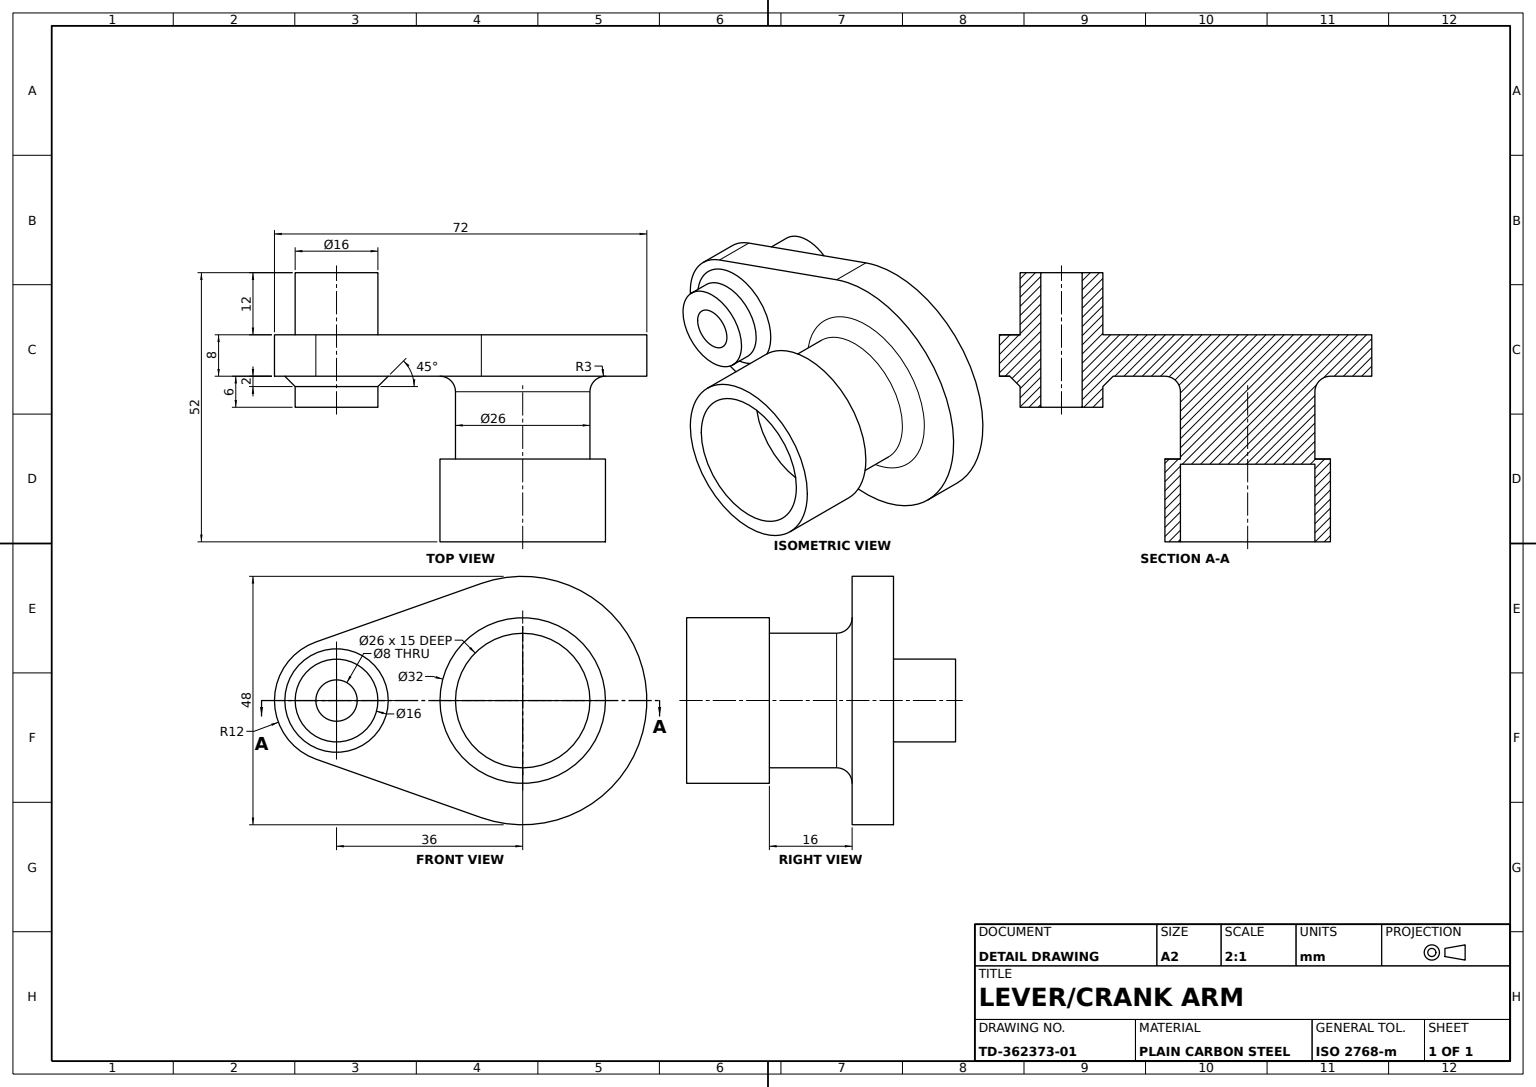
SolidWorks part; units mm, degrees
material "Plain Carbon Steel"
ref_plane "Front Plane" through (0, 0, 0) normal (0, 0, 1) x (1, 0, 0)
ref_plane "Top Plane" through (0, 0, 0) normal (0, 1, 0) x (1, 0, 0)
ref_plane "Right Plane" through (0, 0, 0) normal (1, 0, 0) x (0, 0, -1)
sketch "Oval Plate Sketch" plane through (0, 0, 0) normal (0, 0, 1) x (1, 0, 0)
  line L0 (0, 0) -> (-36, 0)
  line L1 (-40, 11.3137) -> (-8, 22.6274)
  line L2 (-40, -11.3137) -> (-8, -22.6274)
  arc A0 (-8, -22.6274) -> (-8, 22.6274) centre (0, 0) ccw
  arc A1 (-40, 11.3137) -> (-40, -11.3137) centre (-36, 0) ccw
  dimension "D1" = 24
  dimension "D3" = 12
  dimension "D2" = 36
extrude "Oval Plate" add sketch "Oval Plate Sketch" along normal blind 8
sketch "Pin Boss Sketch" plane through (0, 0, 8) normal (0, 0, 1) x (1, 0, 0)
  circle A0 centre (-36, 0) radius 8
  dimension "D1" = 8
extrude "Pin Boss" add sketch "Pin Boss Sketch" along normal blind 6
sketch "Rear Boss Sketch" plane through (0, 0, 0) normal (0, 0, -1) x (-1, 0, 0)
  circle A0 centre (36, 0) radius 8
  dimension "D1" = 16
extrude "Rear Boss" add sketch "Rear Boss Sketch" along normal blind 12
sketch "Tube Neck Sketch" plane through (0, 0, 8) normal (0, 0, 1) x (1, 0, 0)
  circle A0 centre (0, 0) radius 13
  dimension "D1" = 26
extrude "Tube Neck Ø26" add sketch "Tube Neck Sketch" along normal blind 16
sketch "Tube Boss Sketch" plane through (0, 0, 24) normal (0, 0, 1) x (1, 0, 0)
  circle A0 centre (0, 0) radius 16
  dimension "D1" = 32
extrude "Tube Boss Ø32" add sketch "Tube Boss Sketch" along normal blind 16
sketch "Tube Bore Sketch" plane through (0, 0, 40) normal (0, 0, 1) x (1, 0, 0)
  circle A0 centre (0, 0) radius 13
  dimension "D1" = 26
extrude "Tube Bore Ø26" cut sketch "Tube Bore Sketch" against normal blind 15
fillet "Tube Neck Root Fillet R3" radius 3 1 edges at (13, 0, 8)
chamfer "Pin Boss Chamfer 2mm" distance 2 angle 45 1 edges at (-28, 0, 8)
sketch "Pin Hole Sketch" plane through (0, 0, 14) normal (0, 0, 1) x (1, 0, 0)
  circle A0 centre (-36, 0) radius 4
  dimension "D1" = 8
extrude "Pin Through Hole" cut sketch "Pin Hole Sketch" against normal blind 50
